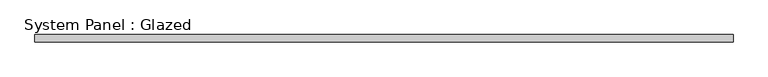
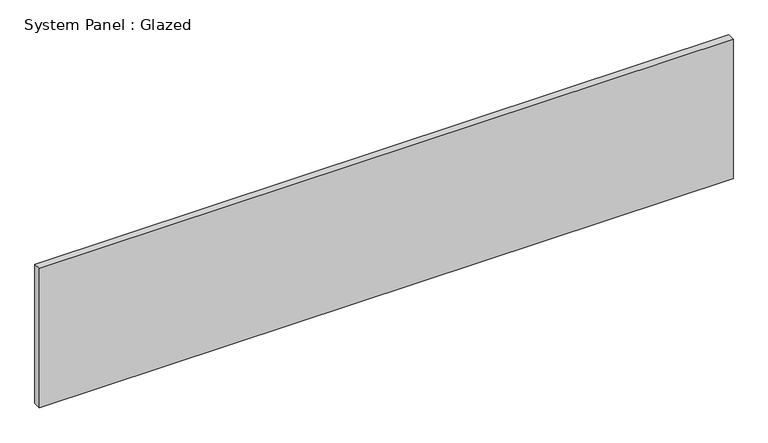
"""IFC4 building model written with IfcOpenShell, lengths in millimetres: plate geometry, System Panel : Glazed."""

from ifc_helpers import new_model, si_unit, origin, origin_with_axes, place, context, project, spatial, polyline, outline, extrude, source, transform, mapped, element, save


def system_panel_glazed_93d7cfd2(model_context):
    return source(origin(), model_context, "Body", "SweptSolid", [
        extrude(outline(polyline([(1171.575, 19.05), (-1171.575, 19.05), (-1171.575, 44.45), (1171.575, 44.45), (1171.575, 19.05)])), origin_with_axes(), (0.0, 0.0, 1.0), 497.405826),
    ])


if __name__ == "__main__":
    model = new_model("IFC4")
    model_context = context("Model", 3, world=origin())
    ifc_project = project(units=[si_unit("LENGTHUNIT", "METRE", prefix="MILLI")], contexts=[model_context])
    site = spatial("IfcSite", under=ifc_project)
    building = spatial("IfcBuilding", under=site)
    placement = place(None, origin())
    system_panel_glazed_shape = system_panel_glazed_93d7cfd2(model_context)
    element("IfcPlate", 1, ObjectType="System Panel : Glazed", at=placement, inside=building, context=model_context, shape_type="MappedRepresentation", body=[
        mapped(system_panel_glazed_shape, transform((0.0, 0.0, 0.0), x_axis=(1.0, 0.0, 0.0), y_axis=(0.0, 1.0, 0.0), z_axis=(0.0, 0.0, 1.0))),
    ])
    save(model, "model.ifc")

# Revit data of these elements
# Type "System Panel : Glazed"
#   Construction Type Id = "GSP4R"
#   Analytic Construction = "1/8 in Pilkington single glazing"
#   Visual Light Transmittance = 0.9
#   Solar Heat Gain Coefficient = 0.86
#   Heat Transfer Coefficient (U) = 1.18115 BTU/(h·ft²·°F)
#   Define Thermal Properties by = 1
# Element 1 (IfcPlate, "System Panel : Glazed")
#   Materials on its faces: "Glass"
# Materials
#   "Glass": class "Glass", colour RGB 0 128 192, transparency 0.75, Description = "Soda Lime Glass", Cost = 0
